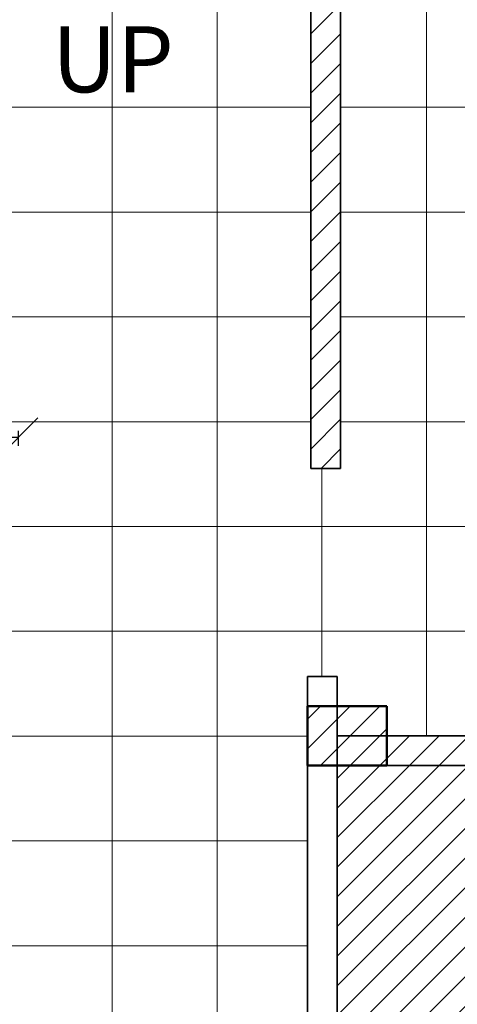
# Model space of a CAD drawing. Units: inches. Extents: x 2036 to 2670, y 319 to 920.
# Tile 7 of 15: x 2383 to 2449, y 579 to 728. Entities that reach past the tile are written whole.
import ezdxf

# ---------------------------------------------------------------- set-up
doc = ezdxf.new("R2010")
doc.units = ezdxf.units.IN
for name, color, linetype, lineweight in [('A-ANNO-DIMS', 2, 'Continuous', 18), ('A-ANNO-TEXT', 7, 'Continuous', 18), ('A-CASE-PATT', 9, 'Continuous', 13), ('A-COLS', 7, 'Continuous', 50), ('A-FLOR-PATT', 8, 'Continuous', 9), ('A-WALL', 7, 'Continuous', 35)]:
    doc.layers.add(name, color=color, linetype=linetype, lineweight=lineweight)
doc.layers.add('A-COLS-PATT', color=240, linetype='Continuous', lineweight=13, true_color=0xed1f24)
doc.layers.add('A-WALL-PATT', color=52, linetype='Continuous', lineweight=13, true_color=0xc8c92d)
doc.styles.get("Standard").update_dxf_attribs({"font": 'arial.ttf'})
doc.dimstyles.new('ISO-25', dxfattribs={"dimtxt": 10, "dimasz": 6, "dimexe": 1.25, "dimexo": 0.625, "dimtad": 0, "dimdec": 1, "dimlunit": 3, "dimtxsty": 'Standard', "dimblk": 'OBLIQUE', "dimcen": 2.5, "dimclrd": 94, "dimclre": 94, "dimclrt": 1, "dimadec": 0, "dimazin": 0, "dimtfac": 1, "dimtdec": 1, "dimtmove": 0, "dimatfit": 3, "dimfxl": 1, "dimfxlon": 1, "dimarcsym": 0})

# ---------------------------------------------------------------- blocks, each defined once
blk = doc.blocks.new('COL-9x12')
blk.add_lwpolyline([(9, 0), (0, 0), (0, 12), (9, 12)], close=True)
blk = doc.blocks.new('_Oblique')
at = {"color": 0, "linetype": 'ByBlock', "lineweight": -2}
blk.add_line((-0.5, -0.5), (0.5, 0.5), dxfattribs=at)
blk = doc.blocks.new('*D40')
at = {"layer": 'A-ANNO-DIMS', "color": 94, "lineweight": -2, "transparency": 16777216}
for p, q in [((2327.86, 665.36), (2327.86, 663.11)), ((2382.86, 665.36), (2382.86, 663.11)), ((2327.86, 664.36), (2341.24, 664.36)), ((2382.86, 664.36), (2369.48, 664.36))]:
    blk.add_line(p, q, dxfattribs=at)
at = {"layer": 'Defpoints', "color": 0, "transparency": 16777216}
for p in [(2327.86, 678.01), (2382.86, 678.01), (2382.86, 664.36)]:
    blk.add_point(p, dxfattribs=at)
at = {"layer": 'A-ANNO-DIMS', "color": 94, "lineweight": -2, "transparency": 16777216, "xscale": 6, "yscale": 6, "zscale": 6, "rotation": 180}
blk.add_blockref('_Oblique', (2327.86, 664.36), dxfattribs=at)
at = {"layer": 'A-ANNO-DIMS', "color": 94, "lineweight": -2, "transparency": 16777216, "xscale": 6, "yscale": 6, "zscale": 6}
blk.add_blockref('_Oblique', (2382.86, 664.36), dxfattribs=at)
at = {"layer": 'A-ANNO-DIMS', "color": 1, "transparency": 16777216, "insert": (2355.36, 664.36), "char_height": 10, "attachment_point": 5}
blk.add_mtext('4\'-7"', dxfattribs=at)
blk = doc.blocks.new('*D54')
at = {"layer": 'A-ANNO-DIMS', "color": 94, "lineweight": -2, "transparency": 16777216}
for p, q in [((2642.09, 545.51), (2642.09, 551.51)), ((2641.09, 545.51), (2643.34, 545.51)), ((2642.09, 513.19), (2642.09, 545.51)), ((2641.09, 513.19), (2643.34, 513.19))]:
    blk.add_line(p, q, dxfattribs=at)
at = {"layer": 'Defpoints', "color": 0, "transparency": 16777216}
for p in [(2158.74, 545.51), (2642.09, 545.51), (2158.74, 513.19)]:
    blk.add_point(p, dxfattribs=at)
at = {"layer": 'A-ANNO-DIMS', "color": 94, "lineweight": -2, "transparency": 16777216, "xscale": 6, "yscale": 6, "zscale": 6}
for p, rotation in [((2642.09, 545.51), 90), ((2642.09, 513.19), 270)]:
    blk.add_blockref('_Oblique', p, dxfattribs=dict(at, rotation=rotation))
at = {"layer": 'A-ANNO-DIMS', "color": 1, "transparency": 16777216, "insert": (2642.09, 577.16), "char_height": 10, "attachment_point": 5, "rotation": 90}
blk.add_mtext('2\'-8 1/2"', dxfattribs=at)
blk = doc.blocks.new('*D55')
at = {"layer": 'A-ANNO-DIMS', "color": 94, "lineweight": -2, "transparency": 16777216}
for p, q in [((2641.09, 582.53), (2643.34, 582.53)), ((2642.09, 582.53), (2642.09, 577.94)), ((2642.09, 545.51), (2642.09, 550.11)), ((2641.09, 545.51), (2643.34, 545.51))]:
    blk.add_line(p, q, dxfattribs=at)
at = {"layer": 'Defpoints', "color": 0, "transparency": 16777216}
for p in [(2158.74, 582.53), (2642.09, 582.53), (2158.74, 545.51)]:
    blk.add_point(p, dxfattribs=at)
at = {"layer": 'A-ANNO-DIMS', "color": 94, "lineweight": -2, "transparency": 16777216, "xscale": 6, "yscale": 6, "zscale": 6}
for p, rotation in [((2642.09, 582.53), 90), ((2642.09, 545.51), 270)]:
    blk.add_blockref('_Oblique', p, dxfattribs=dict(at, rotation=rotation))
at = {"layer": 'A-ANNO-DIMS', "color": 1, "transparency": 16777216, "insert": (2642.09, 564.02), "char_height": 10, "attachment_point": 5, "rotation": 90}
blk.add_mtext('3\'-1"', dxfattribs=at)
blk = doc.blocks.new('*D56')
at = {"layer": 'A-ANNO-DIMS', "color": 94, "lineweight": -2, "transparency": 16777216}
for p, q in [((2642.09, 599.85), (2642.09, 605.85)), ((2641.09, 599.85), (2643.34, 599.85)), ((2642.09, 582.53), (2642.09, 599.85)), ((2641.09, 582.53), (2643.34, 582.53))]:
    blk.add_line(p, q, dxfattribs=at)
at = {"layer": 'Defpoints', "color": 0, "transparency": 16777216}
for p in [(2158.74, 599.85), (2642.09, 599.85), (2158.74, 582.53)]:
    blk.add_point(p, dxfattribs=at)
at = {"layer": 'A-ANNO-DIMS', "color": 94, "lineweight": -2, "transparency": 16777216, "xscale": 6, "yscale": 6, "zscale": 6}
for p, rotation in [((2642.09, 599.85), 90), ((2642.09, 582.53), 270)]:
    blk.add_blockref('_Oblique', p, dxfattribs=dict(at, rotation=rotation))
at = {"layer": 'A-ANNO-DIMS', "color": 1, "transparency": 16777216, "insert": (2642.09, 630.95), "char_height": 10, "attachment_point": 5, "rotation": 90}
blk.add_mtext('1\'-5 1/2"', dxfattribs=at)
blk = doc.blocks.new('*D57')
at = {"layer": 'A-ANNO-DIMS', "color": 94, "lineweight": -2, "transparency": 16777216}
for p, q in [((2642.09, 659.68), (2642.09, 665.68)), ((2641.09, 659.68), (2643.34, 659.68)), ((2642.09, 628.18), (2642.09, 659.68)), ((2641.09, 628.18), (2643.34, 628.18))]:
    blk.add_line(p, q, dxfattribs=at)
at = {"layer": 'Defpoints', "color": 0, "transparency": 16777216}
for p in [(2427.24, 659.68), (2642.09, 659.68), (2426.74, 628.18)]:
    blk.add_point(p, dxfattribs=at)
at = {"layer": 'A-ANNO-DIMS', "color": 94, "lineweight": -2, "transparency": 16777216, "xscale": 6, "yscale": 6, "zscale": 6}
for p, rotation in [((2642.09, 659.68), 90), ((2642.09, 628.18), 270)]:
    blk.add_blockref('_Oblique', p, dxfattribs=dict(at, rotation=rotation))
at = {"layer": 'A-ANNO-DIMS', "color": 1, "transparency": 16777216, "insert": (2642.09, 691.34), "char_height": 10, "attachment_point": 5, "rotation": 90}
blk.add_mtext('2\'-7 1/2"', dxfattribs=at)
blk = doc.blocks.new('*D59')
at = {"layer": 'A-ANNO-DIMS', "color": 94, "lineweight": -2, "transparency": 16777216}
for p, q in [((2641.09, 714.81), (2643.34, 714.81)), ((2642.09, 714.81), (2642.09, 710.72)), ((2642.09, 678.81), (2642.09, 682.89)), ((2641.09, 678.81), (2643.34, 678.81))]:
    blk.add_line(p, q, dxfattribs=at)
at = {"layer": 'Defpoints', "color": 0, "transparency": 16777216}
for p in [(2235.24, 714.81), (2642.09, 714.81), (2235.24, 678.81)]:
    blk.add_point(p, dxfattribs=at)
at = {"layer": 'A-ANNO-DIMS', "color": 94, "lineweight": -2, "transparency": 16777216, "xscale": 6, "yscale": 6, "zscale": 6}
for p, rotation in [((2642.09, 714.81), 90), ((2642.09, 678.81), 270)]:
    blk.add_blockref('_Oblique', p, dxfattribs=dict(at, rotation=rotation))
at = {"layer": 'A-ANNO-DIMS', "color": 1, "transparency": 16777216, "insert": (2642.09, 696.81), "char_height": 10, "attachment_point": 5, "rotation": 90}
blk.add_mtext('3\'-0"', dxfattribs=at)
blk = doc.blocks.new('*D60')
at = {"layer": 'A-ANNO-DIMS', "color": 94, "lineweight": -2, "transparency": 16777216}
for p, q in [((2051.39, 582.41), (2051.39, 588.41)), ((2052.39, 582.41), (2050.14, 582.41)), ((2051.39, 545.09), (2051.39, 582.41)), ((2052.39, 545.09), (2050.14, 545.09))]:
    blk.add_line(p, q, dxfattribs=at)
at = {"layer": 'Defpoints', "color": 0, "transparency": 16777216}
for p in [(2051.39, 582.41), (2515.24, 582.41), (2515.24, 545.09)]:
    blk.add_point(p, dxfattribs=at)
at = {"layer": 'A-ANNO-DIMS', "color": 94, "lineweight": -2, "transparency": 16777216, "xscale": 6, "yscale": 6, "zscale": 6}
for p, rotation in [((2051.39, 582.41), 90), ((2051.39, 545.09), 270)]:
    blk.add_blockref('_Oblique', p, dxfattribs=dict(at, rotation=rotation))
at = {"layer": 'A-ANNO-DIMS', "color": 1, "transparency": 16777216, "insert": (2051.39, 613.98), "char_height": 10, "attachment_point": 5, "rotation": 90}
blk.add_mtext('3\'-1 1/2"', dxfattribs=at)

msp = doc.modelspace()

# ---------------------------------------------------------------- hatches: boundary and pattern name
at = {"layer": 'A-CASE-PATT'}
h = msp.add_hatch(dxfattribs=at)
h.set_pattern_fill('ANSI31', color=256)
h.paths.add_polyline_path([(2455.24, 614.68), (2431.24, 614.68), (2431.24, 503.68), (2515.24, 503.68), (2515.24, 527.68), (2455.24, 527.68)])
at = {"layer": 'A-COLS-PATT'}
h = msp.add_hatch(dxfattribs=at)
h.set_pattern_fill('ANSI31', color=256)
h.paths.add_polyline_path([(2089.74, 875.68), (2080.74, 875.68), (2080.74, 863.68), (2089.74, 863.68)])
h.paths.add_polyline_path([(2089.74, 821.68), (2080.74, 821.68), (2080.74, 809.68), (2089.74, 809.68)])
h.paths.add_polyline_path([(2089.74, 624.2), (2080.74, 624.2), (2080.74, 612.2), (2089.74, 612.2)])
h.paths.add_polyline_path([(2158.74, 506.68), (2149.74, 506.68), (2149.74, 494.68), (2158.74, 494.68)])
h.paths.add_polyline_path([(2158.74, 617.33), (2149.74, 617.33), (2149.74, 605.33), (2158.74, 605.33)])
h.paths.add_polyline_path([(2158.74, 736.18), (2149.74, 736.18), (2149.74, 724.18), (2158.74, 724.18)])
h.paths.add_polyline_path([(2158.74, 852.81), (2149.74, 852.81), (2149.74, 843.81), (2158.74, 843.81)])
h.paths.add_polyline_path([(2161.74, 852.81), (2158.74, 852.81), (2158.74, 843.81), (2161.74, 843.81)])
h.paths.add_polyline_path([(2295.21, 857.66), (2290.74, 857.66), (2290.74, 848.68), (2295.21, 848.68)])
h.paths.add_polyline_path([(2290.74, 857.66), (2283.21, 857.66), (2283.21, 848.66), (2290.74, 848.66)])
h.paths.add_polyline_path([(2443.62, 857.68), (2431.62, 857.68), (2431.62, 848.68), (2443.62, 848.68)])
h.paths.add_polyline_path([(2561.81, 857.68), (2549.81, 857.68), (2549.81, 848.68), (2561.81, 848.68)])
h.paths.add_polyline_path([(2295.24, 737.65), (2290.74, 737.65), (2290.74, 728.68), (2295.24, 728.68)])
h.paths.add_polyline_path([(2309.27, 612.12), (2297.27, 612.12), (2297.27, 603.12), (2309.27, 603.12)])
h.paths.add_polyline_path([(2282.24, 503.68), (2270.24, 503.68), (2270.24, 494.68), (2282.24, 494.68)])
h.paths.add_polyline_path([(2431.74, 746.09), (2427.24, 746.09), (2427.24, 737.09), (2431.74, 737.09)])
h.paths.add_polyline_path([(2439.24, 746.09), (2431.74, 746.09), (2431.74, 737.09), (2439.24, 737.09)])
h.paths.add_polyline_path([(2596.59, 736.59), (2584.59, 736.59), (2584.59, 727.59), (2596.59, 727.59)])
h.paths.add_polyline_path([(2586.39, 623.71), (2574.39, 623.71), (2574.39, 619.18), (2586.39, 619.18)])
h.paths.add_polyline_path([(2586.39, 619.18), (2574.39, 619.18), (2574.39, 614.71), (2586.39, 614.71)])
h.paths.add_polyline_path([(2438.74, 623.68), (2431.24, 623.68), (2431.24, 619.18), (2438.74, 619.18)])
h.paths.add_polyline_path([(2438.74, 619.18), (2431.24, 619.18), (2431.24, 614.68), (2438.74, 614.68)])
h.paths.add_polyline_path([(2431.24, 623.68), (2426.74, 623.68), (2426.74, 614.68), (2431.24, 614.68), (2431.24, 619.18)])
h.paths.add_polyline_path([(2527.24, 503.68), (2515.24, 503.68), (2515.24, 494.68), (2527.24, 494.68)])
h.paths.add_polyline_path([(2590.31, 503.68), (2578.31, 503.68), (2578.31, 494.68), (2590.31, 494.68)])
at = {"layer": 'A-FLOR-PATT'}
h = msp.add_hatch(dxfattribs=at)
h.set_pattern_fill('ANSI31', color=256, scale=5, angle=135)
h.paths.add_polyline_path([(2290.74, 659.68), (2158.74, 659.68), (2158.74, 582.53), (2158.74, 545.51), (2158.74, 503.68), (2426.74, 503.68), (2426.74, 614.68), (2426.74, 623.68), (2426.74, 628.18), (2431.24, 628.18), (2431.24, 623.68), (2438.74, 623.68), (2438.74, 619.18), (2574.39, 619.18), (2574.39, 623.71), (2586.39, 623.71), (2586.39, 619.18), (2603.74, 619.18), (2603.74, 824.68), (2431.74, 824.68), (2431.74, 746.09), (2439.24, 746.09), (2439.24, 737.09), (2431.74, 737.09), (2431.74, 659.68), (2427.24, 659.68), (2427.24, 739.48), (2383.24, 739.48), (2383.24, 804.68), (2339.24, 804.68), (2339.24, 749.08), (2295.24, 749.08), (2295.24, 737.65), (2295.27, 737.65), (2295.27, 728.65), (2295.21, 728.65, -0.586418), (2272.74, 728.68), (2272.74, 824.68), (2270.11, 824.68), (2270.11, 829.18), (2290.74, 829.18), (2290.74, 848.66), (2283.21, 848.66), (2283.21, 857.66), (2289.74, 857.66), (2289.74, 874.68), (2158.74, 874.68), (2158.74, 852.81), (2161.74, 852.81), (2161.74, 843.81), (2158.74, 843.81), (2158.74, 829.18), (2224.74, 829.18), (2224.74, 800.68), (2182.74, 800.68), (2182.74, 733.41), (2158.74, 733.41), (2158.74, 728.68), (2235.24, 728.68), (2235.24, 714.81), (2230.74, 714.81), (2230.74, 724.18), (2158.74, 724.18), (2158.74, 664.18), (2230.74, 664.18), (2230.74, 678.81), (2235.24, 678.81), (2235.24, 664.18), (2290.74, 664.18)])
h.paths.add_polyline_path([(2309.27, 612.12), (2309.27, 603.12), (2297.27, 603.12), (2297.27, 612.12)], flags=16)
h.paths.add_polyline_path([(2280.12, 639.11), (2280.26, 638.18, -0.414214), (2279.26, 637.18), (2278.76, 637.18), (2279.26, 633.18), (2277.76, 633.18), (2277.26, 637.18), (2269.76, 637.18), (2262.26, 637.18), (2261.76, 633.18), (2260.26, 633.18), (2260.76, 637.18), (2260.26, 637.18, -0.414214), (2259.26, 638.18), (2259.41, 639.11, -0.541164), (2257.76, 641.18), (2260.76, 652.18), (2261.45, 652.18), (2261.53, 652.68), (2262.76, 652.68), (2262.25, 655.24, 0.001913), (2261.76, 655.18), (2259.76, 658.18, -0.15), (2279.76, 658.18), (2277.76, 655.18, 0.001913), (2277.27, 655.24), (2276.76, 652.68), (2278, 652.68), (2278.07, 652.18), (2278.76, 652.18), (2281.76, 641.18, -0.541163)], flags=16)
h.paths.add_polyline_path([(2245.98, 639.11), (2246.13, 638.18, -0.414214), (2245.13, 637.18), (2244.63, 637.18), (2245.13, 633.18), (2243.63, 633.18), (2243.13, 637.18), (2235.63, 637.18), (2228.13, 637.18), (2227.63, 633.18), (2226.13, 633.18), (2226.63, 637.18), (2226.13, 637.18, -0.414214), (2225.13, 638.18), (2225.27, 639.11, -0.541164), (2223.63, 641.18), (2226.63, 652.18), (2227.32, 652.18), (2227.39, 652.68), (2228.63, 652.68), (2228.12, 655.24, 0.001913), (2227.63, 655.18), (2225.63, 658.18, -0.15), (2245.63, 658.18), (2243.63, 655.18, 0.001913), (2243.14, 655.24), (2242.63, 652.68), (2243.86, 652.68), (2243.94, 652.18), (2244.63, 652.18), (2247.63, 641.18, -0.541163)], flags=16)
h.paths.add_polyline_path([(2351.59, 515.15, -0.151948), (2279.59, 515.15), (2279.59, 537.68), (2273.59, 537.68), (2273.59, 511.68, 0.190476), (2357.59, 511.68), (2357.59, 537.68), (2351.59, 537.68)])
h.paths.add_polyline_path([(2327.59, 536.13), (2327.59, 517.07), (2303.59, 517.07), (2303.59, 536.13)], flags=16)
h.paths.add_polyline_path([(2213.4, 639.11), (2213.55, 638.18, -0.414214), (2212.55, 637.18), (2212.05, 637.18), (2212.55, 633.18), (2211.05, 633.18), (2210.55, 637.18), (2203.05, 637.18), (2195.55, 637.18), (2195.05, 633.18), (2193.55, 633.18), (2194.05, 637.18), (2193.55, 637.18, -0.414214), (2192.55, 638.18), (2192.69, 639.11, -0.541164), (2191.05, 641.18), (2194.05, 652.18), (2194.73, 652.18), (2194.81, 652.68), (2196.05, 652.68), (2195.53, 655.24, 0.001913), (2195.05, 655.18), (2193.05, 658.18, -0.15), (2213.05, 658.18), (2211.05, 655.18, 0.001913), (2210.56, 655.24), (2210.05, 652.68), (2211.28, 652.68), (2211.36, 652.18), (2212.05, 652.18), (2215.05, 641.18, -0.541163)], flags=16)
h.paths.add_polyline_path([(2368.58, 538.02), (2370.52, 538.02), (2371.17, 532.84), (2380.89, 532.84), (2390.6, 532.84), (2391.25, 538.02), (2393.2, 538.02), (2392.55, 532.84), (2380.89, 532.84), (2368.58, 532.84, 0.414214), (2367.28, 531.54), (2367.47, 530.34, -0.483352), (2369.23, 527.65), (2371.82, 513.4), (2370.12, 513.4), (2370.22, 512.75), (2391.56, 512.75), (2391.66, 513.4), (2389.96, 513.4), (2392.55, 527.65, -1.387427), (2396.43, 527.65), (2392.55, 513.4), (2391.66, 513.4), (2391.56, 512.75), (2389.31, 512.75), (2390, 509.37, 0.003796), (2391.25, 509.51), (2393.84, 505.63, -0.15), (2367.93, 505.63), (2370.52, 509.51, 0.003901), (2371.81, 509.36), (2372.47, 512.75), (2370.22, 512.75), (2370.12, 513.4), (2369.23, 513.4), (2365.34, 527.65, -0.541163), (2367.47, 530.34), (2367.28, 531.54, -0.414214), (2368.58, 532.84), (2369.23, 532.84)])
h.paths.add_polyline_path([(2266.74, 538.02), (2266.09, 532.84), (2254.43, 532.84), (2242.12, 532.84, 0.414214), (2240.83, 531.54), (2241.01, 530.34, -0.483352), (2242.77, 527.65), (2245.36, 513.4), (2243.66, 513.4), (2243.76, 512.75), (2265.1, 512.75), (2265.2, 513.4), (2263.5, 513.4), (2266.09, 527.65, -1.387427), (2269.98, 527.65), (2266.09, 513.4), (2265.2, 513.4), (2265.1, 512.75), (2262.85, 512.75), (2263.54, 509.37, 0.003796), (2264.79, 509.51), (2267.39, 505.63, -0.15), (2241.47, 505.63), (2244.07, 509.51, 0.003901), (2245.36, 509.36), (2246.01, 512.75), (2243.76, 512.75), (2243.66, 513.4), (2242.77, 513.4), (2238.88, 527.65, -0.541163), (2241.01, 530.34), (2240.83, 531.54, -0.414214), (2242.12, 532.84), (2242.77, 532.84), (2242.12, 538.02), (2244.07, 538.02), (2244.71, 532.84), (2254.43, 532.84), (2264.15, 532.84), (2264.79, 538.02)])
h.paths.add_polyline_path([(2185.24, 620.36), (2185.24, 618.86), (2181.24, 618.36), (2181.24, 610.86), (2181.24, 603.36), (2185.24, 602.86), (2185.24, 601.36), (2181.24, 601.86), (2181.24, 601.36, -0.414214), (2180.24, 600.36), (2179.31, 600.5, -0.541164), (2177.24, 598.86), (2166.24, 601.86), (2166.24, 602.54), (2165.74, 602.62), (2165.74, 603.86), (2163.18, 603.34, 0.001913), (2163.24, 602.86), (2160.24, 600.86, -0.15), (2160.24, 620.86), (2163.24, 618.86, 0.001913), (2163.18, 618.37), (2165.74, 617.86), (2165.74, 619.09), (2166.24, 619.17), (2166.24, 619.86), (2177.24, 622.86, -0.541163), (2179.31, 621.21), (2180.24, 621.36, -0.414214), (2181.24, 620.36), (2181.24, 619.86)])
h.paths.add_polyline_path([(2470.92, 676.01), (2470.92, 806.13), (2568.52, 806.13), (2568.52, 676.01)], flags=16)
h.paths.add_polyline_path([(2177.74, 677.49), (2161.9, 677.49), (2161.9, 705.85), (2177.74, 705.85)], flags=16)
h.paths.add_polyline_path([(2176.74, 678.49), (2162.9, 678.49), (2162.9, 704.85), (2176.74, 704.85)], flags=0)
h.paths.add_polyline_path([(2175.01, 686.48), (2172.93, 686.48), (2172.93, 690.63), (2170.86, 690.63), (2170.86, 686.48), (2164.63, 686.48), (2164.63, 688.56), (2166.71, 688.56), (2168.78, 688.56), (2168.78, 690.63), (2164.63, 690.63), (2164.63, 696.85), (2166.71, 696.85), (2166.71, 692.71), (2168.78, 692.71), (2168.78, 696.85), (2175.01, 696.85), (2175.01, 694.78), (2170.86, 694.78), (2170.86, 692.71), (2175.01, 692.71)], flags=0)
h.paths.add_polyline_path([(2543.79, 782.71), (2483.94, 782.71), (2483.94, 804.18), (2517.77, 804.18), (2517.77, 782.71), (2521.67, 782.71), (2521.67, 804.18), (2555.5, 804.18), (2555.5, 779.45), (2547.05, 779.45), (2568.52, 757.98), (2543.79, 757.98)], flags=0)
h.paths.add_polyline_path([(2584.59, 727.59), (2584.59, 736.59), (2596.59, 736.59), (2596.59, 727.59)], flags=16)
h.paths.add_polyline_path([(2520.45, 647.03), (2553.79, 647.03), (2553.79, 658.23), (2520.45, 658.23)], flags=24)
h.paths.add_polyline_path([(2299.53, 573.74), (2331.71, 573.74), (2331.71, 584.94), (2299.53, 584.94)], flags=24)
h.paths.add_polyline_path([(2191.59, 685.19), (2212.12, 685.19), (2212.12, 696.38), (2191.59, 696.38)], flags=24)
h.paths.add_polyline_path([(2353.9, 649.86), (2379.08, 649.86), (2379.08, 661.06), (2353.9, 661.06)], flags=24)
h.paths.add_polyline_path([(2214.61, 763.31), (2237.46, 763.31), (2237.46, 779.56), (2214.61, 779.56)], flags=24)
h.paths.add_polyline_path([(2225.09, 819.31), (2269.29, 819.31), (2269.29, 844.04), (2225.09, 844.04)], flags=24)
h.paths.add_polyline_path([(2204.06, 845.04), (2226.92, 845.04), (2226.92, 856.24), (2204.06, 856.24)], flags=24)
h = msp.add_hatch(dxfattribs=at)
h.set_pattern_fill('ANSI31', color=256, scale=5, angle=45)
h.paths.add_polyline_path([(2290.74, 659.68), (2158.74, 659.68), (2158.74, 582.53), (2158.74, 545.51), (2158.74, 503.68), (2426.74, 503.68), (2426.74, 614.68), (2426.74, 623.68), (2426.74, 628.18), (2431.24, 628.18), (2431.24, 623.68), (2438.74, 623.68), (2438.74, 619.18), (2574.39, 619.18), (2574.39, 623.71), (2586.39, 623.71), (2586.39, 619.18), (2603.74, 619.18), (2603.74, 824.68), (2431.74, 824.68), (2431.74, 746.09), (2439.24, 746.09), (2439.24, 737.09), (2431.74, 737.09), (2431.74, 659.68), (2427.24, 659.68), (2427.24, 739.48), (2383.24, 739.48), (2383.24, 804.68), (2339.24, 804.68), (2339.24, 749.08), (2295.24, 749.08), (2295.24, 737.65), (2295.27, 737.65), (2295.27, 728.65), (2295.21, 728.65, -0.586418), (2272.74, 728.68), (2272.74, 824.68), (2270.11, 824.68), (2270.11, 829.18), (2290.74, 829.18), (2290.74, 848.66), (2283.21, 848.66), (2283.21, 857.66), (2289.74, 857.66), (2289.74, 874.68), (2158.74, 874.68), (2158.74, 852.81), (2161.74, 852.81), (2161.74, 843.81), (2158.74, 843.81), (2158.74, 829.18), (2224.74, 829.18), (2224.74, 800.68), (2182.74, 800.68), (2182.74, 733.41), (2158.74, 733.41), (2158.74, 728.68), (2235.24, 728.68), (2235.24, 714.81), (2230.74, 714.81), (2230.74, 724.18), (2158.74, 724.18), (2158.74, 664.18), (2230.74, 664.18), (2230.74, 678.81), (2235.24, 678.81), (2235.24, 664.18), (2290.74, 664.18)])
h.paths.add_polyline_path([(2309.27, 612.12), (2309.27, 603.12), (2297.27, 603.12), (2297.27, 612.12)], flags=16)
h.paths.add_polyline_path([(2280.12, 639.11), (2280.26, 638.18, -0.414214), (2279.26, 637.18), (2278.76, 637.18), (2279.26, 633.18), (2277.76, 633.18), (2277.26, 637.18), (2269.76, 637.18), (2262.26, 637.18), (2261.76, 633.18), (2260.26, 633.18), (2260.76, 637.18), (2260.26, 637.18, -0.414214), (2259.26, 638.18), (2259.41, 639.11, -0.541164), (2257.76, 641.18), (2260.76, 652.18), (2261.45, 652.18), (2261.53, 652.68), (2262.76, 652.68), (2262.25, 655.24, 0.001913), (2261.76, 655.18), (2259.76, 658.18, -0.15), (2279.76, 658.18), (2277.76, 655.18, 0.001913), (2277.27, 655.24), (2276.76, 652.68), (2278, 652.68), (2278.07, 652.18), (2278.76, 652.18), (2281.76, 641.18, -0.541163)], flags=16)
h.paths.add_polyline_path([(2245.98, 639.11), (2246.13, 638.18, -0.414214), (2245.13, 637.18), (2244.63, 637.18), (2245.13, 633.18), (2243.63, 633.18), (2243.13, 637.18), (2235.63, 637.18), (2228.13, 637.18), (2227.63, 633.18), (2226.13, 633.18), (2226.63, 637.18), (2226.13, 637.18, -0.414214), (2225.13, 638.18), (2225.27, 639.11, -0.541164), (2223.63, 641.18), (2226.63, 652.18), (2227.32, 652.18), (2227.39, 652.68), (2228.63, 652.68), (2228.12, 655.24, 0.001913), (2227.63, 655.18), (2225.63, 658.18, -0.15), (2245.63, 658.18), (2243.63, 655.18, 0.001913), (2243.14, 655.24), (2242.63, 652.68), (2243.86, 652.68), (2243.94, 652.18), (2244.63, 652.18), (2247.63, 641.18, -0.541163)], flags=16)
h.paths.add_polyline_path([(2351.59, 537.68), (2351.59, 515.15, -0.151948), (2279.59, 515.15), (2279.59, 537.68), (2273.59, 537.68), (2273.59, 511.68, 0.190476), (2357.59, 511.68), (2357.59, 537.68)])
h.paths.add_polyline_path([(2368.58, 538.02), (2370.52, 538.02), (2371.17, 532.84), (2380.89, 532.84), (2390.6, 532.84), (2391.25, 538.02), (2393.2, 538.02), (2392.55, 532.84), (2380.89, 532.84), (2368.58, 532.84, 0.414214), (2367.28, 531.54), (2367.47, 530.34, -0.483352), (2369.23, 527.65), (2371.82, 513.4), (2370.12, 513.4), (2370.22, 512.75), (2391.56, 512.75), (2391.66, 513.4), (2389.96, 513.4), (2392.55, 527.65, -1.387427), (2396.43, 527.65), (2392.55, 513.4), (2391.66, 513.4), (2391.56, 512.75), (2389.31, 512.75), (2390, 509.37, 0.003796), (2391.25, 509.51), (2393.84, 505.63, -0.15), (2367.93, 505.63), (2370.52, 509.51, 0.003901), (2371.81, 509.36), (2372.47, 512.75), (2370.22, 512.75), (2370.12, 513.4), (2369.23, 513.4), (2365.34, 527.65, -0.541163), (2367.47, 530.34), (2367.28, 531.54, -0.414214), (2368.58, 532.84), (2369.23, 532.84)])
h.paths.add_polyline_path([(2327.59, 536.13), (2327.59, 517.07), (2303.59, 517.07), (2303.59, 536.13)], flags=16)
h.paths.add_polyline_path([(2470.92, 676.01), (2470.92, 806.13), (2568.52, 806.13), (2568.52, 676.01)], flags=16)
h.paths.add_polyline_path([(2266.74, 538.02), (2266.09, 532.84), (2254.43, 532.84), (2242.12, 532.84, 0.414214), (2240.83, 531.54), (2241.01, 530.34, -0.483352), (2242.77, 527.65), (2245.36, 513.4), (2243.66, 513.4), (2243.76, 512.75), (2265.1, 512.75), (2265.2, 513.4), (2263.5, 513.4), (2266.09, 527.65, -1.387427), (2269.98, 527.65), (2266.09, 513.4), (2265.2, 513.4), (2265.1, 512.75), (2262.85, 512.75), (2263.54, 509.37, 0.003796), (2264.79, 509.51), (2267.39, 505.63, -0.15), (2241.47, 505.63), (2244.07, 509.51, 0.003901), (2245.36, 509.36), (2246.01, 512.75), (2243.76, 512.75), (2243.66, 513.4), (2242.77, 513.4), (2238.88, 527.65, -0.541163), (2241.01, 530.34), (2240.83, 531.54, -0.414214), (2242.12, 532.84), (2242.77, 532.84), (2242.12, 538.02), (2244.07, 538.02), (2244.71, 532.84), (2254.43, 532.84), (2264.15, 532.84), (2264.79, 538.02)])
h.paths.add_polyline_path([(2213.4, 639.11), (2213.55, 638.18, -0.414214), (2212.55, 637.18), (2212.05, 637.18), (2212.55, 633.18), (2211.05, 633.18), (2210.55, 637.18), (2203.05, 637.18), (2195.55, 637.18), (2195.05, 633.18), (2193.55, 633.18), (2194.05, 637.18), (2193.55, 637.18, -0.414214), (2192.55, 638.18), (2192.69, 639.11, -0.541164), (2191.05, 641.18), (2194.05, 652.18), (2194.73, 652.18), (2194.81, 652.68), (2196.05, 652.68), (2195.53, 655.24, 0.001913), (2195.05, 655.18), (2193.05, 658.18, -0.15), (2213.05, 658.18), (2211.05, 655.18, 0.001913), (2210.56, 655.24), (2210.05, 652.68), (2211.28, 652.68), (2211.36, 652.18), (2212.05, 652.18), (2215.05, 641.18, -0.541163)], flags=16)
h.paths.add_polyline_path([(2185.24, 620.36), (2185.24, 618.86), (2181.24, 618.36), (2181.24, 610.86), (2181.24, 603.36), (2185.24, 602.86), (2185.24, 601.36), (2181.24, 601.86), (2181.24, 601.36, -0.414214), (2180.24, 600.36), (2179.31, 600.5, -0.541164), (2177.24, 598.86), (2166.24, 601.86), (2166.24, 602.54), (2165.74, 602.62), (2165.74, 603.86), (2163.18, 603.34, 0.001913), (2163.24, 602.86), (2160.24, 600.86, -0.15), (2160.24, 620.86), (2163.24, 618.86, 0.001913), (2163.18, 618.37), (2165.74, 617.86), (2165.74, 619.09), (2166.24, 619.17), (2166.24, 619.86), (2177.24, 622.86, -0.541163), (2179.31, 621.21), (2180.24, 621.36, -0.414214), (2181.24, 620.36), (2181.24, 619.86)])
h.paths.add_polyline_path([(2177.74, 677.49), (2161.9, 677.49), (2161.9, 705.85), (2177.74, 705.85)], flags=16)
h.paths.add_polyline_path([(2176.74, 678.49), (2162.9, 678.49), (2162.9, 704.85), (2176.74, 704.85)], flags=0)
h.paths.add_polyline_path([(2175.01, 686.48), (2172.93, 686.48), (2172.93, 690.63), (2170.86, 690.63), (2170.86, 686.48), (2164.63, 686.48), (2164.63, 688.56), (2166.71, 688.56), (2168.78, 688.56), (2168.78, 690.63), (2164.63, 690.63), (2164.63, 696.85), (2166.71, 696.85), (2166.71, 692.71), (2168.78, 692.71), (2168.78, 696.85), (2175.01, 696.85), (2175.01, 694.78), (2170.86, 694.78), (2170.86, 692.71), (2175.01, 692.71)], flags=0)
h.paths.add_polyline_path([(2543.79, 782.71), (2483.94, 782.71), (2483.94, 804.18), (2517.77, 804.18), (2517.77, 782.71), (2521.67, 782.71), (2521.67, 804.18), (2555.5, 804.18), (2555.5, 779.45), (2547.05, 779.45), (2568.52, 757.98), (2543.79, 757.98)], flags=0)
h.paths.add_polyline_path([(2584.59, 727.59), (2584.59, 736.59), (2596.59, 736.59), (2596.59, 727.59)], flags=16)
h.paths.add_polyline_path([(2520.45, 647.03), (2553.79, 647.03), (2553.79, 658.23), (2520.45, 658.23)], flags=24)
h.paths.add_polyline_path([(2299.53, 573.74), (2331.71, 573.74), (2331.71, 584.94), (2299.53, 584.94)], flags=24)
h.paths.add_polyline_path([(2191.59, 685.19), (2212.12, 685.19), (2212.12, 696.38), (2191.59, 696.38)], flags=24)
h.paths.add_polyline_path([(2353.9, 649.86), (2379.08, 649.86), (2379.08, 661.06), (2353.9, 661.06)], flags=24)
h.paths.add_polyline_path([(2214.61, 763.31), (2237.46, 763.31), (2237.46, 779.56), (2214.61, 779.56)], flags=24)
h.paths.add_polyline_path([(2225.09, 819.31), (2269.29, 819.31), (2269.29, 844.04), (2225.09, 844.04)], flags=24)
h.paths.add_polyline_path([(2204.06, 845.04), (2226.92, 845.04), (2226.92, 856.24), (2204.06, 856.24)], flags=24)
h = msp.add_hatch(dxfattribs=at)
h.set_pattern_fill('ANSI31', color=256, scale=3, angle=135)
h.paths.add_polyline_path([(2149.74, 582.53), (2149.74, 707.68), (2120.74, 707.68), (2120.74, 599.68, -1), (2118.74, 599.68), (2085.24, 599.68), (2085.24, 506.68), (2089.74, 506.68), (2089.74, 494.68), (2085.24, 494.68), (2085.24, 469.18), (2608.24, 469.18), (2608.24, 494.68), (2149.74, 494.68), (2149.74, 506.68), (2149.74, 545.51)])
h.paths.add_polyline_path([(2143.58, 686.71), (2149.03, 686.71), (2149.03, 692.89), (2143.58, 692.89)], flags=24)
h.paths.add_polyline_path([(2125.99, 700.31), (2133.31, 700.31), (2133.31, 706.49), (2125.99, 706.49)], flags=24)
at = {"layer": 'A-WALL-PATT'}
h = msp.add_hatch(dxfattribs=at)
h.set_pattern_fill('ANSI31', color=256)
h.paths.add_polyline_path([(2089.74, 863.68), (2080.74, 863.68), (2080.74, 821.68), (2089.74, 821.68)])
h.paths.add_polyline_path([(2089.74, 809.68), (2080.74, 809.68), (2080.74, 624.2), (2089.74, 624.2), (2089.74, 707.68), (2089.74, 767.68)])
h.paths.add_polyline_path([(2149.74, 818.68), (2089.74, 818.68), (2089.74, 809.68), (2149.74, 809.68)])
h.paths.add_polyline_path([(2158.74, 875.68), (2089.74, 875.68), (2089.74, 866.68), (2149.74, 866.68), (2149.74, 852.81), (2158.74, 852.81)])
h.paths.add_polyline_path([(2158.74, 843.81), (2149.74, 843.81), (2149.74, 736.18), (2158.74, 736.18), (2158.74, 824.68)])
h.paths.add_polyline_path([(2181.31, 829.18), (2158.74, 829.18), (2158.74, 824.68), (2181.31, 824.68)])
h.paths.add_polyline_path([(2224.74, 829.18), (2212.72, 829.18), (2212.72, 824.68), (2224.74, 824.68)])
h.paths.add_polyline_path([(2177.02, 503.68), (2158.74, 503.68), (2158.74, 494.68), (2177.02, 494.68)])
h.paths.add_polyline_path([(2158.74, 664.18), (2158.74, 680.02), (2149.74, 680.02), (2149.74, 617.33), (2158.74, 617.33)])
h.paths.add_polyline_path([(2158.74, 724.18), (2149.74, 724.18), (2149.74, 704.02), (2158.74, 704.02)])
h.paths.add_polyline_path([(2235.24, 728.68), (2158.74, 728.68), (2158.74, 724.18), (2230.74, 724.18), (2230.74, 714.81), (2235.24, 714.81)])
h.paths.add_polyline_path([(2290.74, 664.18), (2235.24, 664.18), (2235.24, 678.81), (2230.74, 678.81), (2230.74, 664.18), (2158.74, 664.18), (2158.74, 659.68), (2290.74, 659.68)])
h.paths.add_polyline_path([(2270.24, 503.68), (2227.17, 503.68), (2227.17, 494.68), (2270.24, 494.68)])
h.paths.add_polyline_path([(2515.24, 503.68), (2380.89, 503.68), (2380.89, 494.68), (2515.24, 494.68)])
h.paths.add_polyline_path([(2292.21, 503.68), (2282.24, 503.68), (2282.24, 494.68), (2292.21, 494.68)])
h.paths.add_polyline_path([(2578.31, 503.68), (2527.24, 503.68), (2527.24, 494.68), (2578.31, 494.68)])
h.paths.add_polyline_path([(2603.74, 503.68), (2590.31, 503.68), (2590.31, 494.68), (2603.74, 494.68)])
h.paths.add_polyline_path([(2612.74, 503.68), (2603.74, 503.68), (2603.74, 494.68), (2612.74, 494.68)])
h.paths.add_polyline_path([(2549.81, 857.68), (2443.62, 857.68), (2443.62, 848.68), (2549.81, 848.68)])
h.paths.add_polyline_path([(2295.24, 848.66), (2290.74, 848.66), (2290.74, 829.18), (2270.11, 829.18), (2270.11, 824.68), (2290.74, 824.68), (2290.74, 737.65), (2295.24, 737.65)])
h.paths.add_polyline_path([(2431.74, 737.09), (2427.24, 737.09), (2427.24, 659.68), (2431.74, 659.68)])
h.paths.add_polyline_path([(2431.74, 848.68), (2427.24, 848.68), (2427.24, 746.09), (2431.74, 746.09)])
h.paths.add_polyline_path([(2574.39, 619.18), (2495.46, 619.18), (2495.46, 614.68), (2574.39, 614.68)])
h.paths.add_polyline_path([(2461.84, 619.18), (2438.74, 619.18), (2438.74, 614.68), (2461.84, 614.68)])
h.paths.add_polyline_path([(2603.74, 619.18), (2586.39, 619.18), (2586.39, 614.68), (2603.74, 614.68)], flags=17)

# ---------------------------------------------------------------- linework, layer by layer
at = {"layer": 'A-WALL'}
for p, q in [((2427.24, 659.68), (2427.24, 848.68)), ((2431.74, 659.68), (2431.74, 848.68)), ((2427.24, 659.68), (2431.74, 659.68)), ((2426.74, 623.68), (2426.74, 628.18)), ((2426.74, 628.18), (2431.24, 628.18)), ((2431.24, 614.68), (2431.24, 628.18)), ((2426.74, 614.68), (2426.74, 623.68)), ((2603.74, 619.18), (2431.24, 619.18)), ((2426.74, 503.68), (2426.74, 614.68)), ((2603.74, 614.68), (2431.24, 614.68)), ((2431.24, 503.68), (2431.24, 614.68))]:
    msp.add_line(p, q, dxfattribs=at)

# ---------------------------------------------------------------- block references
at = {"layer": 'A-COLS', "rotation": 89.9999999999986}
msp.add_blockref('COL-9x12', (2438.74, 614.68), dxfattribs=at)

# ---------------------------------------------------------------- texts
at = {"layer": 'A-ANNO-TEXT', "insert": (2387.99, 726.65), "char_height": 10, "attachment_point": 1}
msp.add_mtext_dynamic_manual_height_columns('UP', width=32.758, gutter_width=12.5, heights=[0], dxfattribs=at)

# ---------------------------------------------------------------- dimensions: what is measured, and where the dimension line sits
at = {"layer": 'A-ANNO-DIMS'}
for base, p1, p2, picture, middle in [((2642.09, 714.81), (2235.24, 678.81), (2235.24, 714.81), '*D59', (2642.09, 696.81)), ((2642.09, 659.68), (2426.74, 628.18), (2427.24, 659.68), '*D57', (2642.09, 691.34)), ((2642.09, 599.85), (2158.74, 582.53), (2158.74, 599.85), '*D56', (2642.09, 630.95)), ((2051.39, 582.41), (2515.24, 545.09), (2515.24, 582.41), '*D60', (2051.39, 613.98)), ((2642.09, 545.51), (2158.74, 513.19), (2158.74, 545.51), '*D54', (2642.09, 577.16)), ((2642.09, 582.53), (2158.74, 545.51), (2158.74, 582.53), '*D55', (2642.09, 564.02))]:
    dim = msp.add_linear_dim(base=base, p1=p1, p2=p2, angle=90, dimstyle='ISO-25', override={"dimdec": 1, "dimlfac": 1, "dimrnd": 0, "dimzin": 1, "dimdsep": 46, "dimlunit": 4, "dimfrac": 2}, dxfattribs=at)
    dim.commit()
    dim.dimension.update_dxf_attribs({"geometry": picture, "text_midpoint": middle})
dim = msp.add_linear_dim(base=(2382.86, 664.36), p1=(2327.86, 678.01), p2=(2382.86, 678.01), dimstyle='ISO-25', override={"dimdec": 1, "dimlfac": 1, "dimrnd": 0, "dimzin": 1, "dimdsep": 46, "dimlunit": 4, "dimfrac": 2}, dxfattribs=at)
dim.commit()
dim.dimension.update_dxf_attribs({"geometry": '*D40', "text_midpoint": (2355.36, 664.36)})

doc.saveas('drawing.dxf')
